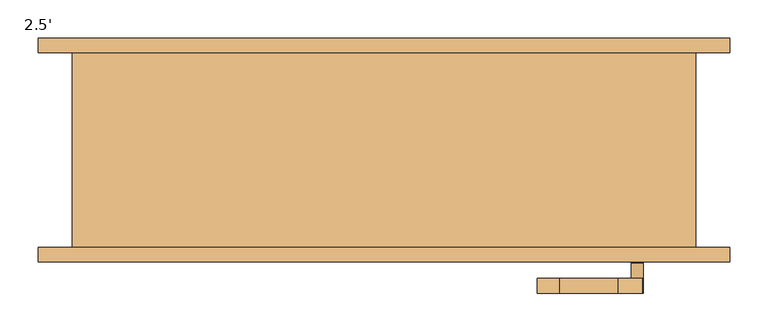
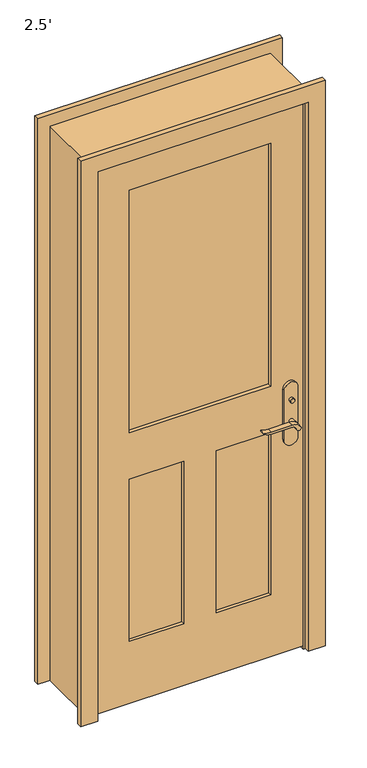
"""IFC4 building model written with IfcOpenShell, lengths in millimetres: door geometry, 2.5'."""

from ifc_helpers import new_model, si_unit, point, frame, frame_2d, origin, place, context, project, spatial, polyline, circle_curve, trimmed, segment, composite_curve, outline, extrude, faceted_brep, source, transform, mapped, element, save


def door_2_5_90776985(model_context):
    return source(origin(), model_context, "Body", "SolidModel", [
        extrude(outline(polyline([(-38.1, 12.7), (-12.7, 0.0), (-98.425, 0.0), (-73.025, 12.7), (-38.1, 12.7)])), frame((-381.0, 0.0, 0.0), z_axis=(1.0, 0.0, 0.0), x_axis=(0.0, 1.0, 0.0)), (0.0, 0.0, 1.0), 762.0),
        extrude(outline(polyline([(335.2, -68.9), (335.2, -78.9), (325.2, -78.9), (325.2, -68.9), (335.2, -68.9)])), frame((0.0, 0.0, 981.9), z_axis=(0.0, 0.0, 1.0), x_axis=(1.0, 0.0, 0.0)), (0.0, 0.0, 1.0), 30.0),
        extrude(outline(composite_curve([segment(trimmed(circle_curve(frame_2d((996.9, 330.2)), 8.0), [point((996.9, 322.2))], [point((996.9, 338.2))], False, "CARTESIAN"), True, "CONTINUOUS"), segment(trimmed(circle_curve(frame_2d((996.9, 330.2)), 8.0), [point((996.9, 338.2))], [point((996.9, 322.2))], False, "CARTESIAN"), True, "CONTINUOUS")], self_intersect=False)), frame((0.0, -143.825, 0.0), z_axis=(0.0, 1.0, 0.0), x_axis=(0.0, 0.0, 1.0)), (0.0, 0.0, 1.0), 10.0),
        extrude(outline(composite_curve([segment(trimmed(circle_curve(frame_2d((897.1555521, 306.5324871)), 37.2832219), [point((919.0523287, 336.7081363))], [point((934.4, 304.8325667))], False, "CARTESIAN"), True, "CONTINUOUS"), segment(polyline([(934.4, 304.8325667), (934.4, 228.5564091)]), True, "CONTINUOUS"), segment(trimmed(circle_curve(frame_2d((1017.6850638, 228.6227909)), 83.2850902), [point((934.4, 228.5564091))], [point((939.4, 200.2))], True, "CARTESIAN"), True, "CONTINUOUS"), segment(polyline([(939.4, 200.2), (936.6135558, 200.2)]), True, "CONTINUOUS"), segment(trimmed(circle_curve(frame_2d((986.6709207, 232.1396612)), 59.3791355), [point((936.6135558, 200.2))], [point((927.4, 228.5564091))], False, "CARTESIAN"), True, "CONTINUOUS"), segment(polyline([(927.4, 228.5564091), (927.4, 304.8138099)]), True, "CONTINUOUS"), segment(trimmed(circle_curve(frame_2d((909.2738613, 304.8138099)), 18.1261387), [point((927.4, 304.8138099))], [point((914.4, 322.2))], True, "CARTESIAN"), True, "CONTINUOUS"), segment(trimmed(circle_curve(frame_2d((914.4, 330.2)), 8.0), [point((914.4, 322.2))], [point((919.0523287, 336.7081363))], False, "CARTESIAN"), True, "CONTINUOUS")], self_intersect=False)), frame((0.0, -48.9, 0.0), z_axis=(0.0, 1.0, 0.0), x_axis=(0.0, 0.0, 1.0)), (0.0, 0.0, 1.0), 20.0),
        extrude(outline(composite_curve([segment(trimmed(circle_curve(frame_2d((914.4, 330.2)), 8.0), [point((914.3999903, 322.2))], [point((919.0523287, 336.7081363))], False, "CARTESIAN"), True, "CONTINUOUS"), segment(trimmed(circle_curve(frame_2d((897.1555521, 306.5324871)), 37.2832219), [point((919.0523287, 336.7081363))], [point((934.4, 304.8325667))], False, "CARTESIAN"), True, "CONTINUOUS"), segment(polyline([(934.4, 304.8325667), (934.4, 228.5564091)]), True, "CONTINUOUS"), segment(trimmed(circle_curve(frame_2d((1017.6850638, 228.6227909)), 83.2850902), [point((934.4, 228.5564091))], [point((939.4, 200.2))], True, "CARTESIAN"), True, "CONTINUOUS"), segment(polyline([(939.4, 200.2), (936.6135558, 200.2)]), True, "CONTINUOUS"), segment(trimmed(circle_curve(frame_2d((986.6709207, 232.1396612)), 59.3791355), [point((936.6135558, 200.2))], [point((927.4, 228.5564091))], False, "CARTESIAN"), True, "CONTINUOUS"), segment(polyline([(927.4, 228.5564091), (927.4, 304.8138122)]), True, "CONTINUOUS"), segment(trimmed(circle_curve(frame_2d((909.2738682, 304.8138122)), 18.1261318), [point((927.4, 304.8138122))], [point((914.3999903, 322.2))], True, "CARTESIAN"), True, "CONTINUOUS")], self_intersect=False)), frame((0.0, -183.825, 0.0), z_axis=(0.0, 1.0, 0.0), x_axis=(0.0, 0.0, 1.0)), (0.0, 0.0, 1.0), 20.0),
        extrude(outline(composite_curve([segment(trimmed(circle_curve(frame_2d((914.4, 330.2)), 8.0), [point((914.4, 322.2))], [point((914.4, 338.2))], False, "CARTESIAN"), True, "CONTINUOUS"), segment(trimmed(circle_curve(frame_2d((914.4, 330.2)), 8.0), [point((914.4, 338.2))], [point((914.4, 322.2))], False, "CARTESIAN"), True, "CONTINUOUS")], self_intersect=False)), frame((0.0, -78.9, 0.0), z_axis=(0.0, 1.0, 0.0), x_axis=(0.0, 0.0, 1.0)), (0.0, 0.0, 1.0), 30.0),
        extrude(outline(composite_curve([segment(trimmed(circle_curve(frame_2d((914.4, 330.2)), 8.0), [point((914.4, 322.2))], [point((914.4, 338.2))], False, "CARTESIAN"), True, "CONTINUOUS"), segment(trimmed(circle_curve(frame_2d((914.4, 330.2)), 8.0), [point((914.4, 338.2))], [point((914.4, 322.2))], False, "CARTESIAN"), True, "CONTINUOUS")], self_intersect=False)), frame((0.0, -163.825, 0.0), z_axis=(0.0, 1.0, 0.0), x_axis=(0.0, 0.0, 1.0)), (0.0, 0.0, 1.0), 30.0),
        extrude(outline(composite_curve([segment(polyline([(844.4, 355.2), (1039.4, 355.2)]), True, "CONTINUOUS"), segment(trimmed(circle_curve(frame_2d((1039.4, 330.2)), 25.0), [point((1039.4, 355.2))], [point((1039.4, 305.2))], False, "CARTESIAN"), True, "CONTINUOUS"), segment(polyline([(1039.4, 305.2), (844.4, 305.2)]), True, "CONTINUOUS"), segment(trimmed(circle_curve(frame_2d((844.4, 330.2)), 25.0), [point((844.4, 305.2))], [point((844.4, 355.2))], False, "CARTESIAN"), True, "CONTINUOUS")], self_intersect=False)), frame((0.0, -88.9, 0.0), z_axis=(0.0, 1.0, 0.0), x_axis=(0.0, 0.0, 1.0)), (0.0, 0.0, 1.0), 10.0),
        extrude(outline(composite_curve([segment(polyline([(844.4, 355.2), (1039.4, 355.2)]), True, "CONTINUOUS"), segment(trimmed(circle_curve(frame_2d((1039.4, 330.2)), 25.0), [point((1039.4, 355.2))], [point((1039.4, 305.2))], False, "CARTESIAN"), True, "CONTINUOUS"), segment(polyline([(1039.4, 305.2), (844.4, 305.2)]), True, "CONTINUOUS"), segment(trimmed(circle_curve(frame_2d((844.4, 330.2)), 25.0), [point((844.4, 305.2))], [point((844.4, 355.2))], False, "CARTESIAN"), True, "CONTINUOUS")], self_intersect=False)), frame((0.0, -133.825, 0.0), z_axis=(0.0, 1.0, 0.0), x_axis=(0.0, 0.0, 1.0)), (0.0, 0.0, 1.0), 10.0),
        faceted_brep([(406.4, -123.825, 0.0), (381.0, -123.825, 0.0), (381.0, -88.9, 0.0), (368.3, -88.9, 0.0), (368.3, -53.975, 0.0), (381.0, -53.975, 0.0), (381.0, 130.175, 0.0), (406.4, 130.175, 0.0), (406.4, 130.175, 2159.0), (406.4, -123.825, 2159.0), (381.0, 130.175, 2133.6), (-381.0, 130.175, 2133.6), (-381.0, 130.175, 0.0), (-406.4, 130.175, 0.0), (-406.4, 130.175, 2159.0), (381.0, -53.975, 2133.6), (368.3, -53.975, 2120.9), (-368.3, -53.975, 2120.9), (-368.3, -53.975, 0.0), (-381.0, -53.975, 0.0), (-381.0, -53.975, 2133.6), (368.3, -88.9, 2120.9), (381.0, -88.9, 2133.6), (-381.0, -88.9, 2133.6), (-381.0, -88.9, 0.0), (-368.3, -88.9, 0.0), (-368.3, -88.9, 2120.9), (381.0, -123.825, 2133.6), (-406.4, -123.825, 2159.0), (-406.4, -123.825, 0.0), (-381.0, -123.825, 0.0), (-381.0, -123.825, 2133.6)], [[[0, 1, 2, 3, 4, 5, 6, 7]], [[7, 8, 9, 0]], [[6, 10, 11, 12, 13, 14, 8, 7]], [[5, 15, 10, 6]], [[4, 16, 17, 18, 19, 20, 15, 5]], [[3, 21, 16, 4]], [[2, 22, 23, 24, 25, 26, 21, 3]], [[1, 27, 22, 2]], [[0, 9, 28, 29, 30, 31, 27, 1]], [[8, 14, 28, 9]], [[15, 20, 11, 10]], [[21, 26, 17, 16]], [[27, 31, 23, 22]], [[29, 13, 12, 19, 18, 25, 24, 30]], [[14, 13, 29, 28]], [[20, 19, 12, 11]], [[26, 25, 18, 17]], [[31, 30, 24, 23]]]),
        extrude(outline(polyline([(2133.6, -381.0), (12.7, -381.0), (12.7, 381.0), (2133.6, 381.0), (2133.6, -381.0)]), holes=[polyline([(1066.8, -260.35), (2012.95, -260.35), (2012.95, 260.35), (1066.8, 260.35), (1066.8, -260.35)]), polyline([(885.825, -60.325), (254.0, -60.325), (254.0, -260.35), (885.825, -260.35), (885.825, -60.325)]), polyline([(885.825, 260.35), (254.0, 260.35), (254.0, 60.325), (885.825, 60.325), (885.825, 260.35)])]), frame((0.0, -123.825, 0.0), z_axis=(0.0, 1.0, 0.0), x_axis=(0.0, 0.0, 1.0)), (0.0, 0.0, 1.0), 34.925),
        extrude(outline(polyline([(260.35, -102.87), (260.35, -109.855), (-260.35, -109.855), (-260.35, -102.87), (260.35, -102.87)])), frame((0.0, 0.0, 1066.8), z_axis=(0.0, 0.0, 1.0), x_axis=(1.0, 0.0, 0.0)), (0.0, 0.0, 1.0), 946.15),
        extrude(outline(polyline([(-60.325, -100.5416667), (-60.325, -112.1833333), (-260.35, -112.1833333), (-260.35, -100.5416667), (-60.325, -100.5416667)])), frame((0.0, 0.0, 254.0), z_axis=(0.0, 0.0, 1.0), x_axis=(1.0, 0.0, 0.0)), (0.0, 0.0, 1.0), 631.825),
        extrude(outline(polyline([(260.35, -100.5416667), (260.35, -112.1833333), (60.325, -112.1833333), (60.325, -100.5416667), (260.35, -100.5416667)])), frame((0.0, 0.0, 254.0), z_axis=(0.0, 0.0, 1.0), x_axis=(1.0, 0.0, 0.0)), (0.0, 0.0, 1.0), 631.825),
        extrude(outline(polyline([(0.0, -387.35), (2139.95, -387.35), (2139.95, 387.35), (0.0, 387.35), (0.0, 450.85), (2203.45, 450.85), (2203.45, -450.85), (0.0, -450.85), (0.0, -387.35)])), frame((0.0, -142.875, 0.0), z_axis=(0.0, 1.0, 0.0), x_axis=(0.0, 0.0, 1.0)), (0.0, 0.0, 1.0), 19.05),
        extrude(outline(polyline([(0.0, -387.35), (2139.95, -387.35), (2139.95, 387.35), (0.0, 387.35), (0.0, 450.85), (2203.45, 450.85), (2203.45, -450.85), (0.0, -450.85), (0.0, -387.35)])), frame((0.0, 130.175, 0.0), z_axis=(0.0, 1.0, 0.0), x_axis=(0.0, 0.0, 1.0)), (0.0, 0.0, 1.0), 19.05),
    ])


if __name__ == "__main__":
    model = new_model("IFC4")
    model_context = context("Model", 3, world=origin())
    ifc_project = project(units=[si_unit("LENGTHUNIT", "METRE", prefix="MILLI")], contexts=[model_context])
    site = spatial("IfcSite", under=ifc_project)
    building = spatial("IfcBuilding", under=site)
    placement = place(None, origin())
    door_2_5_shape = door_2_5_90776985(model_context)
    element("IfcDoor", 1, ObjectType="2.5'", at=placement, inside=building, context=model_context, shape_type="MappedRepresentation", body=[
        mapped(door_2_5_shape, transform((0.0, 0.0, 0.0), x_axis=(1.0, 0.0, 0.0), y_axis=(0.0, 1.0, 0.0), z_axis=(0.0, 0.0, 1.0))),
    ])
    save(model, "model.ifc")

# Revit data of these elements
# Type "2.5'"
#   Type Mark = "11"
#   Assembly Code = "B2030100"
#   Analytic Construction = "French door, wood frame with single glass"
#   Top Rail = 0' - 4 3/4"
#   Threshold Offset [instance default] = 0' - 0 1/2"
#   Thickness = 0' - 1 3/8"
#   Thermal Resistance (R) = 1.0696 (h·ft²·°F)/BTU
#   Swing Angle [instance default] = 90.00°
#   Stiles = 0' - 4 3/4"
#   Rough Width = 2' - 8"
#   Rough Height = 7' - 1"
#   Lock Rail = 0' - 7 1/8"
#   Height = 7' - 0"
#   Width = 2' - 6"
#   Heat Transfer Coefficient (U) = 0.9350 BTU/(h·ft²·°F)
#   Door Offset [instance default] = 0' - 0"
#   Bottom Rail = 0' - 9 1/2"
#   Threshold [instance default] = yes
#   Function = 1
#   Exterior Trim [instance default] = yes
#   Trim Material = Cherry
#   Threshold Material = Cherry
#   Panel Material = Cherry
#   Glazing = Glass
#   Frame Material = Cherry
#   Door Handle Material = Aluminum
#   Visual Light Transmittance = 0
#   Solar Heat Gain Coefficient = 0
#   Wall Closure = (empty or 0)
#   Construction Type = (empty or 0)
# Element 1 (IfcDoor, "2.5'")
#   Materials on its faces: "Cherry", "Aluminum", "Glass"
# Materials
#   "Cherry": class "Wood", colour RGB 226 177 128, transparency 0, Description = "Prunus Serotina", Cost = 0
#   "Glass": class "Glass", colour RGB 0 128 192, transparency 0.75, Description = "Soda Lime Glass", Cost = 0
#   "Aluminum": class "Metal", colour RGB 247 247 247, transparency 0, Description = "Aluminum 6061", Cost = 0
